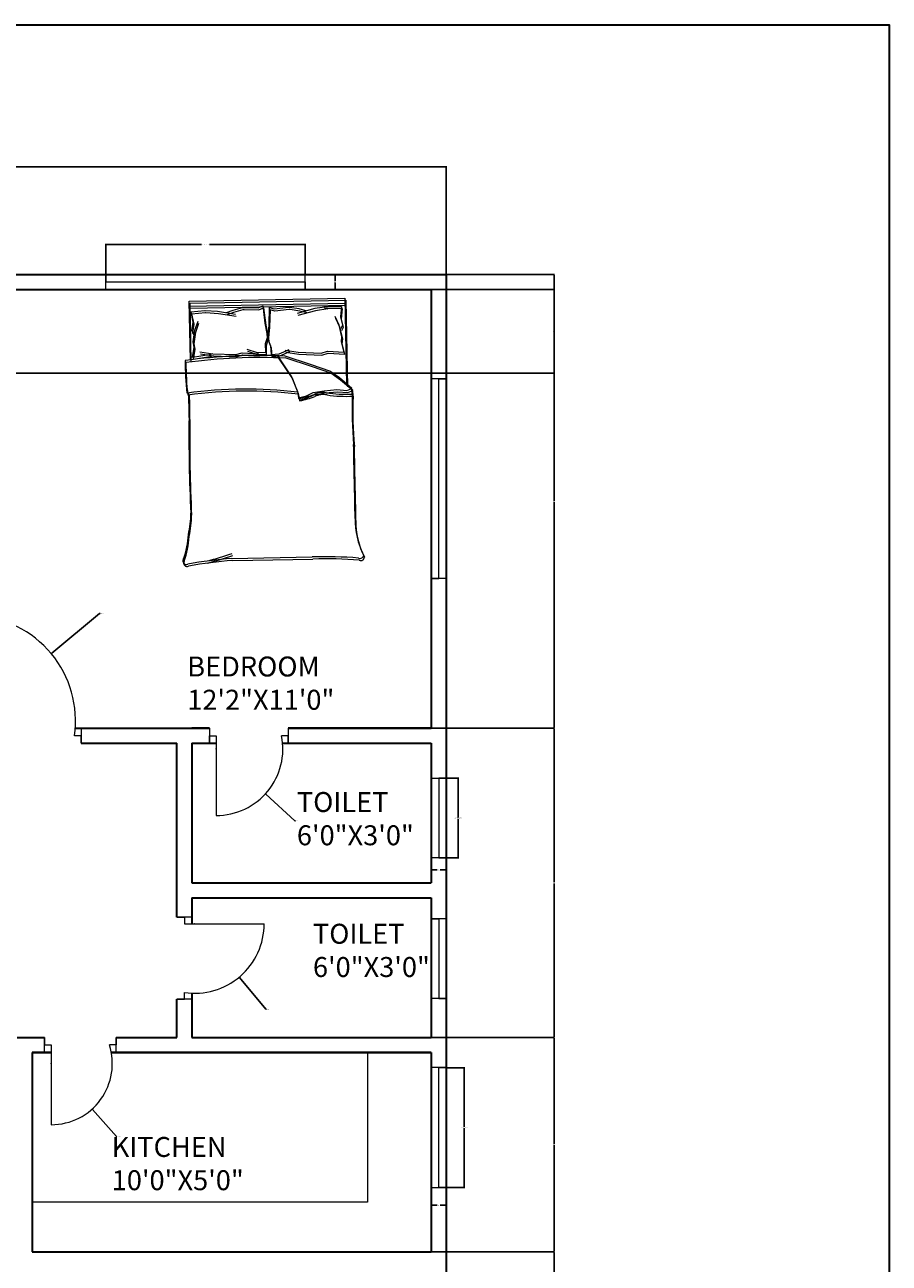
# Model space of a CAD drawing. Units: inches. Extents: x 1721 to 2510, y 1544 to 2360.
# Tile 10 of 10: x 2250 to 2510, y 1988 to 2360. Entities that reach past the tile are written whole.
import ezdxf

# ---------------------------------------------------------------- set-up
doc = ezdxf.new("R2010")
doc.units = ezdxf.units.IN
for name, color, linetype, lineweight in [('A-ANNO-DIMS', 2, 'Continuous', 18), ('A-ANNO-TTLB', 7, 'Continuous', 35), ('A-AREA-IDEN', 7, 'Continuous', 18), ('A-DOOR', 3, 'Continuous', 18), ('A-FLOR-FIXT', 9, 'Continuous', 18), ('A-FURN', 8, 'Continuous', 13), ('A-GLAZ', 4, 'Continuous', 18), ('A-WALL', 7, 'Continuous', 35)]:
    doc.layers.add(name, color=color, linetype=linetype, lineweight=lineweight)
doc.styles.get("Standard").update_dxf_attribs({"font": 'arial.ttf'})
doc.dimstyles.get("Standard").update_dxf_attribs({"dimtxt": 0.18, "dimasz": 0.18, "dimexe": 0.18, "dimexo": 0.0625, "dimgap": 0.09, "dimtad": 0, "dimtih": 1, "dimtoh": 1, "dimdec": 4, "dimzin": 0, "dimdsep": 46, "dimtxsty": 'Standard', "dimcen": 0.09, "dimadec": 0, "dimazin": 0, "dimtfac": 1, "dimtdec": 4, "dimtofl": 0, "dimtmove": 0, "dimatfit": 3, "dimfxl": 1, "dimtolj": 1, "dimtzin": 0, "dimarcsym": 0})

# ---------------------------------------------------------------- blocks, each defined once
blk = doc.blocks.new('BED-DOUBLE')
for p, q in [((39.64, 78.43), (15.52, 78.72)), ((39.64, 78.43), (15.52, 78.72)), ((39.86, 77.8), (15.74, 78.09)), ((39.86, 77.8), (15.74, 78.09)), ((1.93, 30.11), (1.99, 28.4, 3.79)), ((1.93, 30.11), (1.99, 28.4, 3.79)), ((15.66, 30.21), (13.68, 29.32)), ((15.66, 30.21), (13.68, 29.32)), ((18.1, 30.79), (15.66, 30.21)), ((18.1, 30.79), (15.66, 30.21)), ((18.31, 30.16), (15.88, 29.58)), ((18.31, 30.16), (15.88, 29.58)), ((18.38, 28.81), (18.1, 30.79)), ((18.38, 28.81), (18.1, 30.79)), ((18.59, 28.18), (18.31, 30.16)), ((18.59, 28.18), (18.31, 30.16)), ((3.5, 28.99), (1.99, 28.4)), ((3.5, 28.99), (1.99, 28.4)), ((1.99, 28.4), (5.58, 25.17)), ((1.99, 28.4), (5.58, 25.17)), ((2.15, 29.48), (2.21, 27.77, 3.79)), ((2.15, 29.48), (2.21, 27.77, 3.79)), ((3.72, 28.36), (2.21, 27.77)), ((3.72, 28.36), (2.21, 27.77)), ((2.21, 27.77), (5.8, 24.54)), ((2.21, 27.77), (5.8, 24.54)), ((3.23, 1.19), (3.55, 27.27)), ((3.23, 1.19), (3.55, 27.27)), ((3.45, 0.56), (3.76, 26.64)), ((3.45, 0.56), (3.76, 26.64)), ((6.54, 28.65), (3.5, 28.99)), ((6.54, 28.65), (3.5, 28.99)), ((6.75, 28.02), (3.72, 28.36)), ((6.75, 28.02), (3.72, 28.36)), ((10.33, 28.91), (6.54, 28.65)), ((10.33, 28.91), (6.54, 28.65)), ((10.55, 28.28), (6.75, 28.02)), ((10.55, 28.28), (6.75, 28.02)), ((13.68, 29.32), (10.33, 28.91)), ((13.68, 29.32), (10.33, 28.91)), ((13.89, 28.69), (10.55, 28.28)), ((13.89, 28.69), (10.55, 28.28)), ((15.88, 29.58), (13.89, 28.69)), ((15.88, 29.58), (13.89, 28.69)), ((20, 24.39), (18.38, 28.81)), ((20, 24.39), (18.38, 28.81)), ((20.21, 23.76), (18.59, 28.18)), ((20.21, 23.76), (18.59, 28.18)), ((5.58, 25.17), (8.44, 23.01)), ((5.58, 25.17), (8.44, 23.01)), ((5.8, 24.54), (8.66, 22.38)), ((5.8, 24.54), (8.66, 22.38)), ((8.44, 23.01), (13.88, 20.98)), ((8.44, 23.01), (13.88, 20.98)), ((8.66, 22.38), (14.1, 20.35)), ((8.66, 22.38), (14.1, 20.35)), ((24.03, 17.98), (20, 24.39)), ((24.03, 17.98), (20, 24.39)), ((24.24, 17.35), (20.21, 23.76)), ((24.24, 17.35), (20.21, 23.76)), ((13.88, 20.98), (22.02, 18)), ((13.88, 20.98), (22.02, 18)), ((14.1, 20.35), (22.24, 17.37)), ((14.1, 20.35), (22.24, 17.37)), ((9.01, 16.97), (3.98, 17.42)), ((3.98, 17.42), (4.71, 14.34)), ((9.01, 16.97), (3.98, 17.42)), ((3.98, 17.42), (4.71, 14.34)), ((9.23, 16.34), (4.2, 16.8)), ((4.2, 16.8), (4.92, 13.71)), ((9.23, 16.34), (4.2, 16.8)), ((4.2, 16.8), (4.92, 13.71)), ((10.94, 17.49), (9.01, 16.97)), ((10.94, 17.49), (9.01, 16.97)), ((11.15, 16.86), (9.23, 16.34)), ((11.15, 16.86), (9.23, 16.34)), ((17.8, 16.99), (10.94, 17.49)), ((17.8, 16.99), (10.94, 17.49)), ((18.02, 16.36), (11.15, 16.86)), ((18.02, 16.36), (11.15, 16.86)), ((21.75, 16.29), (17.8, 16.99)), ((21.75, 16.29), (17.8, 16.99)), ((21.96, 15.66), (18.02, 16.36)), ((21.96, 15.66), (18.02, 16.36)), ((23.54, 17.35), (20.51, 16.13)), ((23.54, 17.35), (20.51, 16.13)), ((23.75, 16.73), (20.73, 15.5)), ((23.75, 16.73), (20.73, 15.5)), ((25.94, 17.48), (23.54, 17.35)), ((25.94, 17.48), (23.54, 17.35)), ((26.16, 16.85), (23.75, 16.73)), ((26.16, 16.85), (23.75, 16.73)), ((26.07, 14.85), (25.94, 17.48)), ((26.07, 14.85), (25.94, 17.48)), ((26.29, 14.22), (26.16, 16.85)), ((26.29, 14.22), (26.16, 16.85)), ((27.61, 14.21), (27.64, 16.84)), ((27.61, 14.21), (27.64, 16.84)), ((27.64, 16.84), (30.05, 16.81)), ((27.64, 16.84), (30.05, 16.81)), ((27.82, 13.58), (27.85, 16.21)), ((27.82, 13.58), (27.85, 16.21)), ((27.85, 16.21), (30.26, 16.18)), ((27.85, 16.21), (30.26, 16.18)), ((34.67, 16.66), (29.65, 17.12)), ((34.67, 16.66), (29.65, 17.12)), ((34.89, 16.03), (29.86, 16.49)), ((34.89, 16.03), (29.86, 16.49)), ((30.05, 16.81), (33.11, 15.7)), ((30.05, 16.81), (33.11, 15.7)), ((30.26, 16.18), (33.33, 15.07)), ((30.26, 16.18), (33.33, 15.07)), ((36.6, 17.19), (34.67, 16.66)), ((36.6, 17.19), (34.67, 16.66)), ((36.81, 16.56), (34.89, 16.03)), ((36.81, 16.56), (34.89, 16.03)), ((43.46, 16.68), (36.6, 17.19)), ((43.46, 16.68), (36.6, 17.19)), ((43.68, 16.05), (36.81, 16.56)), ((43.68, 16.05), (36.81, 16.56)), ((43.46, 16.68), (44.58, 16.98)), ((43.46, 16.68), (44.58, 16.98)), ((47.41, 15.98), (43.46, 16.68)), ((47.41, 15.98), (43.46, 16.68)), ((43.68, 16.05), (44.79, 16.35)), ((43.68, 16.05), (44.79, 16.35)), ((47.62, 15.35), (43.68, 16.05)), ((47.62, 15.35), (43.68, 16.05)), ((44.58, 16.98), (49.58, 17.63)), ((44.58, 16.98), (49.58, 17.63)), ((44.79, 16.35), (49.8, 17)), ((44.79, 16.35), (49.8, 17)), ((49.58, 17.63), (48.98, 14.52)), ((49.58, 17.63), (48.98, 14.52)), ((49.8, 17), (49.19, 13.89)), ((49.8, 17), (49.19, 13.89)), ((50.28, 18.38), (50.07, 0.63)), ((50.28, 18.38), (50.07, 0.63)), ((50.5, 17.75), (50.29, 0)), ((50.5, 17.75), (50.29, 0)), ((4.71, 14.34), (4.5, 12.77)), ((4.71, 14.34), (4.5, 12.77)), ((4.5, 12.77), (5.25, 9.26)), ((4.5, 12.77), (5.25, 9.26)), ((4.92, 13.71), (4.72, 12.14)), ((4.92, 13.71), (4.72, 12.14)), ((4.72, 12.14), (5.46, 8.63)), ((4.72, 12.14), (5.46, 8.63)), ((26.73, 13.04), (26.07, 14.85)), ((26.73, 13.04), (26.07, 14.85)), ((26.95, 12.41), (26.29, 14.22)), ((26.95, 12.41), (26.29, 14.22)), ((26.39, 8.62), (26.8, 11.77)), ((26.39, 8.62), (26.8, 11.77)), ((26.8, 11.77), (26.73, 13.04)), ((26.8, 11.77), (26.73, 13.04)), ((27.01, 11.14), (26.95, 12.41)), ((27.01, 11.14), (26.95, 12.41)), ((27, 11.1), (27.02, 12.38)), ((27, 11.1), (27.02, 12.38)), ((27.02, 12.38), (27.61, 14.21)), ((27.02, 12.38), (27.61, 14.21)), ((27.22, 10.47), (27.23, 11.75)), ((27.22, 10.47), (27.23, 11.75)), ((27.23, 11.75), (27.82, 13.58)), ((27.23, 11.75), (27.82, 13.58)), ((49.24, 12.96), (48.63, 9.42)), ((49.24, 12.96), (48.63, 9.42)), ((49.46, 12.33), (48.85, 8.79)), ((49.46, 12.33), (48.85, 8.79)), ((48.98, 14.52), (49.24, 12.96)), ((48.98, 14.52), (49.24, 12.96)), ((49.19, 13.89), (49.46, 12.33)), ((49.19, 13.89), (49.46, 12.33)), ((4.25, 9.35), (4.77, 10.37)), ((4.25, 9.35), (4.77, 10.37)), ((4.8, 6.82), (4.25, 9.35)), ((4.8, 6.82), (4.25, 9.35)), ((4.47, 8.72), (4.98, 9.74)), ((4.47, 8.72), (4.98, 9.74)), ((5.02, 6.19), (4.47, 8.72)), ((5.02, 6.19), (4.47, 8.72)), ((5.25, 9.26), (6.37, 6.62)), ((5.25, 9.26), (6.37, 6.62)), ((5.46, 8.63), (6.59, 5.99)), ((5.46, 8.63), (6.59, 5.99)), ((26.09, 3.36), (26.39, 8.62)), ((26.09, 3.36), (26.39, 8.62)), ((26.3, 2.73), (26.61, 7.99)), ((26.3, 2.73), (26.61, 7.99)), ((26.61, 7.99), (27.01, 11.14)), ((26.61, 7.99), (27.01, 11.14)), ((27.53, 7.98), (27, 11.1)), ((27.53, 7.98), (27, 11.1)), ((27.75, 7.35), (27.22, 10.47)), ((27.75, 7.35), (27.22, 10.47)), ((28.04, 2.73), (27.53, 7.98)), ((28.04, 2.73), (27.53, 7.98)), ((48.63, 9.42), (47.61, 6.74)), ((48.63, 9.42), (47.61, 6.74)), ((48.85, 8.79), (47.82, 6.11)), ((48.85, 8.79), (47.82, 6.11)), ((49.63, 9.55), (49.07, 10.55)), ((49.63, 9.55), (49.07, 10.55)), ((49.17, 7.01), (49.63, 9.55)), ((49.17, 7.01), (49.63, 9.55)), ((49.84, 8.92), (49.29, 9.92)), ((49.84, 8.92), (49.29, 9.92)), ((49.39, 6.38), (49.84, 8.92)), ((49.39, 6.38), (49.84, 8.92)), ((4.39, 3.68), (4.8, 6.82)), ((4.39, 3.68), (4.8, 6.82)), ((4.61, 3.05), (5.02, 6.19)), ((4.61, 3.05), (5.02, 6.19)), ((8.71, 3.62), (12.44, 4.09)), ((8.71, 3.62), (12.44, 4.09)), ((12.44, 4.09), (17.76, 5.35)), ((12.44, 4.09), (17.76, 5.35)), ((12.65, 3.46), (17.98, 4.72)), ((12.65, 3.46), (17.98, 4.72)), ((15.1, 4.65), (17.12, 4.04)), ((15.1, 4.65), (17.12, 4.04)), ((15.32, 4.02), (17.34, 3.41)), ((15.32, 4.02), (17.34, 3.41)), ((17.12, 4.04), (19.98, 3.48)), ((17.12, 4.04), (19.98, 3.48)), ((20.3, 3.49), (24.64, 3.85)), ((20.3, 3.49), (24.64, 3.85)), ((24.64, 3.85), (26.09, 3.36)), ((24.64, 3.85), (26.09, 3.36)), ((28.25, 2.1), (27.75, 7.35)), ((28.25, 2.1), (27.75, 7.35)), ((36.97, 3.75), (34.13, 3.08)), ((36.97, 3.75), (34.13, 3.08)), ((41.65, 3.98), (36.28, 5.04)), ((41.65, 3.98), (36.28, 5.04)), ((41.87, 3.35), (36.49, 4.41)), ((41.87, 3.35), (36.49, 4.41)), ((38.96, 4.44), (36.97, 3.75)), ((38.96, 4.44), (36.97, 3.75)), ((39.18, 3.81), (37.19, 3.12)), ((39.18, 3.81), (37.19, 3.12)), ((45.39, 3.65), (41.65, 3.98)), ((45.39, 3.65), (41.65, 3.98)), ((49.7, 3.91), (45.5, 3.63)), ((49.7, 3.91), (45.5, 3.63)), ((49.7, 3.88), (49.17, 7.01)), ((49.7, 3.88), (49.17, 7.01)), ((49.92, 3.25), (49.39, 6.38)), ((49.92, 3.25), (49.39, 6.38)), ((50.07, 0.63), (3.23, 1.19)), ((50.07, 0.63), (3.23, 1.19)), ((50.09, 2.13), (3.25, 2.69)), ((50.09, 2.13), (3.25, 2.69)), ((50.29, 0), (3.45, 0.56)), ((50.29, 0), (3.45, 0.56)), ((50.31, 1.5), (3.47, 2.06)), ((50.31, 1.5), (3.47, 2.06)), ((4.39, 3.68), (9.69, 3.52)), ((4.39, 3.68), (9.69, 3.52)), ((4.61, 3.05), (9.9, 2.89)), ((4.61, 3.05), (9.9, 2.89)), ((9.69, 3.52), (8.71, 3.62)), ((9.69, 3.52), (8.71, 3.62)), ((8.92, 2.99), (12.65, 3.46)), ((8.92, 2.99), (12.65, 3.46)), ((9.9, 2.89), (8.92, 2.99)), ((9.9, 2.89), (8.92, 2.99)), ((17.34, 3.41), (20.2, 2.85)), ((17.34, 3.41), (20.2, 2.85)), ((19.98, 3.48), (20.3, 3.49)), ((19.98, 3.48), (20.3, 3.49)), ((20.2, 2.85), (20.52, 2.86)), ((20.2, 2.85), (20.52, 2.86)), ((20.52, 2.86), (24.86, 3.22)), ((20.52, 2.86), (24.86, 3.22)), ((24.86, 3.22), (26.3, 2.73)), ((24.86, 3.22), (26.3, 2.73)), ((29.46, 3.28), (28.04, 2.73)), ((29.46, 3.28), (28.04, 2.73)), ((29.68, 2.65), (28.25, 2.1)), ((29.68, 2.65), (28.25, 2.1)), ((33.81, 3.08), (29.46, 3.28)), ((33.81, 3.08), (29.46, 3.28)), ((34.03, 2.45), (29.68, 2.65)), ((34.03, 2.45), (29.68, 2.65)), ((34.13, 3.08), (33.81, 3.08)), ((34.13, 3.08), (33.81, 3.08)), ((34.35, 2.45), (34.03, 2.45)), ((34.35, 2.45), (34.03, 2.45)), ((37.19, 3.12), (34.35, 2.45)), ((37.19, 3.12), (34.35, 2.45)), ((45.61, 3.02), (41.87, 3.35)), ((45.61, 3.02), (41.87, 3.35)), ((45.5, 3.63), (45.39, 3.65)), ((45.5, 3.63), (45.39, 3.65)), ((45.71, 3), (45.61, 3.02)), ((45.71, 3), (45.61, 3.02)), ((49.91, 3.28), (45.71, 3)), ((49.91, 3.28), (45.71, 3))]:
    blk.add_line(p, q)
for centre, radius, start, end in [((1.08, 78.52), 1.08, 61.9736, 175.3348), ((1.08, 78.52), 1.08, 61.9736, 175.3348), ((-20.36, 68.78), 22.61, 356.7862, 25.7829), ((-20.36, 68.78), 22.61, 356.7862, 25.7829), ((1.29, 77.89), 1.08, 61.9736, 175.3348), ((1.29, 77.89), 1.08, 61.9736, 175.3348), ((15.63, 209.12), 130.4, 263.8146, 269.9499), ((15.63, 209.12), 130.4, 263.8146, 269.9499), ((15.85, 208.49), 130.4, 263.8146, 269.9499), ((15.85, 208.49), 130.4, 263.8146, 269.9499), ((70.08, -22.85), 104.34, 102.698, 107.0202), ((70.08, -22.85), 104.34, 102.698, 107.0202), ((34.83, 197.67), 119.34, 272.3106, 278.7239), ((34.83, 197.67), 119.34, 272.3106, 278.7239), ((70.29, -23.48), 104.34, 102.698, 107.0202), ((70.29, -23.48), 104.34, 102.698, 107.0202), ((35.05, 197.04), 119.34, 272.3106, 278.7239), ((35.05, 197.04), 119.34, 272.3106, 278.7239), ((53.35, 78.73), 1.07, 325.4884, 112.793), ((53.35, 78.73), 1.07, 325.4884, 112.793), ((53.56, 78.1), 1.07, 325.4884, 112.793), ((53.56, 78.1), 1.07, 325.4884, 112.793), ((-20.14, 68.15), 22.61, 356.7862, 25.7829), ((-20.14, 68.15), 22.61, 356.7862, 25.7829), ((75.53, 69.21), 23.09, 157.2899, 175.9668), ((75.53, 69.21), 23.09, 157.2899, 175.9668), ((75.75, 68.58), 23.09, 157.2899, 175.9668), ((75.75, 68.58), 23.09, 157.2899, 175.9668), ((80.6, 63.5), 29.05, 165.3797, 178.2261), ((80.6, 63.5), 29.05, 165.3797, 178.2261), ((4473.12, 14.21), 4471.22, 179.317, 179.60172), ((4473.12, 14.21), 4471.22, 179.317, 179.60172), ((80.81, 62.87), 29.05, 165.3797, 178.2261), ((80.81, 62.87), 29.05, 165.3797, 178.2261), ((4473.34, 13.58), 4471.22, 179.317, 179.60172), ((4473.34, 13.58), 4471.22, 179.317, 179.60172), ((-421.08, 55.88), 472.73, 357.5425, 1.0334), ((-421.08, 55.88), 472.73, 357.5425, 1.0334), ((-420.87, 55.25), 472.73, 357.5425, 1.0334), ((-420.87, 55.25), 472.73, 357.5425, 1.0334), ((-124.73, 38.32), 126.93, 356.294, 3.1513), ((-124.73, 38.32), 126.93, 356.294, 3.1513), ((-124.51, 37.69), 126.93, 356.294, 3.1513), ((-124.51, 37.69), 126.93, 356.294, 3.1513), ((217.81, 29.18), 166.73, 177.791, 180.323), ((217.81, 29.18), 166.73, 177.791, 180.323), ((218.03, 28.55), 166.73, 177.791, 180.323), ((218.03, 28.55), 166.73, 177.791, 180.323), ((3.1, -5.33), 35.46, 79.1911, 91.8805), ((3.1, -5.33), 35.46, 79.1911, 91.8805), ((11.02, 35.47), 6.1, 257.9756, 293.0532), ((11.02, 35.47), 6.1, 257.9756, 293.0532), ((22.96, 2.41), 29.06, 99.9765, 109.1954), ((22.96, 2.41), 29.06, 99.9765, 109.1954), ((23.18, 1.78), 29.06, 99.9765, 109.1954), ((23.18, 1.78), 29.06, 99.9765, 109.1954), ((17.93, 30.85), 0.181, 339.5612, 90.4525), ((17.93, 30.85), 0.181, 339.5612, 90.4525), ((18.15, 30.22), 0.181, 339.5612, 90.4525), ((18.15, 30.22), 0.181, 339.5612, 90.4525), ((3.31, -5.96), 35.46, 79.1911, 91.8805), ((3.31, -5.96), 35.46, 79.1911, 91.8805), ((11.23, 34.84), 6.1, 257.9756, 293.0532), ((11.23, 34.84), 6.1, 257.9756, 293.0532), ((37.91, 154), 126.46, 261.0993, 276.2154), ((37.91, 154), 126.46, 261.0993, 276.2154), ((38.12, 153.37), 126.46, 261.0993, 276.2154), ((38.12, 153.37), 126.46, 261.0993, 276.2154), ((-29.75, 21.28), 81.65, 358.0366, 4.9188), ((-29.75, 21.28), 81.65, 358.0366, 4.9188), ((-29.53, 20.65), 81.65, 358.0366, 4.9188), ((-29.53, 20.65), 81.65, 358.0366, 4.9188), ((34.68, 179.26), 161.69, 265.4014, 276.097), ((34.68, 179.26), 161.69, 265.4014, 276.097), ((34.89, 178.63), 161.69, 265.4014, 276.097), ((34.89, 178.63), 161.69, 265.4014, 276.097)]:
    blk.add_arc(centre, radius, start, end)
blk = doc.blocks.new('WIN-60IN-A')
for p, q in [((4.5, 60), (0, 60)), ((2.25, 0), (2.25, 60)), ((2.25, 60), (4.5, 60)), ((4.5, 0), (0, 0)), ((0, 0), (2.25, 0))]:
    blk.add_line(p, q)
blk = doc.blocks.new('WIN-24IN-A')
for p, q in [((4.5, 24), (0, 24)), ((0, 24), (2.25, 24)), ((2.25, 24), (2.25, 0)), ((4.5, 0), (0, 0)), ((2.25, 0), (4.5, 0))]:
    blk.add_line(p, q)
blk = doc.blocks.new('WIN-24IN-B')
for p, q in [((0, 24), (4.5, 24)), ((4.5, 24), (2.25, 24)), ((2.25, 24), (2.25, 0)), ((4.5, 0), (0, 0)), ((2.25, 0), (4.5, 0))]:
    blk.add_line(p, q)
blk = doc.blocks.new('WIN-36IN-B')
for p, q in [((4.5, 36), (0, 36)), ((2.25, 0), (2.25, 36)), ((2.25, 36), (4.5, 36)), ((0, 0), (4.5, 0)), ((4.5, 0), (2.25, 0))]:
    blk.add_line(p, q)
blk = doc.blocks.new('*D18')
at = {"layer": 'A-ANNO-DIMS', "color": 0, "lineweight": -2, "transparency": 16777216}
for p, q in [((2274.1, 2285.19), (2274.1, 2294.31)), ((2274.28, 2294.13), (2302.86, 2294.13)), ((2333.92, 2294.13), (2305.33, 2294.13)), ((2334.1, 2285.19), (2334.1, 2294.31))]:
    blk.add_line(p, q, dxfattribs=at)
at = {"layer": 'A-ANNO-DIMS', "color": 0, "transparency": 16777216}
for points in [[(2274.28, 2294.16), (2274.28, 2294.1), (2274.1, 2294.13)], [(2333.92, 2294.16), (2333.92, 2294.1), (2334.1, 2294.13)]]:
    blk.add_solid(points, dxfattribs=at)
at = {"layer": 'Defpoints', "color": 0, "transparency": 16777216}
for p in [(2334.1, 2294.13), (2274.1, 2285.13), (2334.1, 2285.13)]:
    blk.add_point(p, dxfattribs=at)
at = {"layer": 'A-ANNO-DIMS', "color": 0, "transparency": 16777216, "insert": (2304.1, 2294.13), "char_height": 0.18, "attachment_point": 5}
blk.add_mtext('\\A1;WINDOW A 60 TYP.', dxfattribs=at)
blk = doc.blocks.new('*D19')
at = {"layer": 'A-ANNO-DIMS', "color": 0, "lineweight": -2, "transparency": 16777216}
for p, q in [((2334.16, 2285.13), (2343.28, 2285.13)), ((2343.1, 2284.95), (2343.1, 2283.06)), ((2334.16, 2280.63), (2343.28, 2280.63)), ((2343.1, 2280.81), (2343.1, 2282.7))]:
    blk.add_line(p, q, dxfattribs=at)
at = {"layer": 'A-ANNO-DIMS', "color": 0, "transparency": 16777216}
for points in [[(2343.07, 2284.95), (2343.13, 2284.95), (2343.1, 2285.13)], [(2343.07, 2280.81), (2343.13, 2280.81), (2343.1, 2280.63)]]:
    blk.add_solid(points, dxfattribs=at)
at = {"layer": 'Defpoints', "color": 0, "transparency": 16777216}
for p in [(2334.1, 2285.13), (2334.1, 2280.63), (2343.1, 2280.63)]:
    blk.add_point(p, dxfattribs=at)
at = {"layer": 'A-ANNO-DIMS', "color": 0, "transparency": 16777216, "insert": (2343.1, 2282.88), "char_height": 0.18, "attachment_point": 5}
blk.add_mtext('\\A1;5 TYP.', dxfattribs=at)
blk = doc.blocks.new('*D24')
at = {"layer": 'A-ANNO-DIMS', "color": 0, "lineweight": -2, "transparency": 16777216}
for p, q in [((2376.56, 2046.53), (2382.08, 2046.53)), ((2381.9, 2046.35), (2381.9, 2028.72)), ((2381.9, 2010.71), (2381.9, 2028.35)), ((2376.56, 2010.53), (2382.08, 2010.53))]:
    blk.add_line(p, q, dxfattribs=at)
at = {"layer": 'A-ANNO-DIMS', "color": 0, "transparency": 16777216}
for points in [[(2381.87, 2046.35), (2381.93, 2046.35), (2381.9, 2046.53)], [(2381.87, 2010.71), (2381.93, 2010.71), (2381.9, 2010.53)]]:
    blk.add_solid(points, dxfattribs=at)
at = {"layer": 'Defpoints', "color": 0, "transparency": 16777216}
for p in [(2376.5, 2046.53), (2381.9, 2046.53), (2376.5, 2010.53)]:
    blk.add_point(p, dxfattribs=at)
at = {"layer": 'A-ANNO-DIMS', "color": 0, "transparency": 16777216, "insert": (2381.9, 2028.53), "char_height": 0.18, "attachment_point": 5}
blk.add_mtext('\\A1;WINDOW B 36 TYP.', dxfattribs=at)
blk = doc.blocks.new('*D25')
at = {"layer": 'A-ANNO-DIMS', "color": 0, "lineweight": -2, "transparency": 16777216}
for p, q in [((2372, 2010.47), (2372, 2004.95)), ((2376.5, 2010.47), (2376.5, 2004.95)), ((2372.18, 2005.13), (2373.79, 2005.13)), ((2376.32, 2005.13), (2374.71, 2005.13))]:
    blk.add_line(p, q, dxfattribs=at)
at = {"layer": 'A-ANNO-DIMS', "color": 0, "transparency": 16777216}
for points in [[(2372.18, 2005.16), (2372.18, 2005.1), (2372, 2005.13)], [(2376.32, 2005.16), (2376.32, 2005.1), (2376.5, 2005.13)]]:
    blk.add_solid(points, dxfattribs=at)
at = {"layer": 'Defpoints', "color": 0, "transparency": 16777216}
for p in [(2372, 2010.53), (2376.5, 2010.53), (2376.5, 2005.13)]:
    blk.add_point(p, dxfattribs=at)
at = {"layer": 'A-ANNO-DIMS', "color": 0, "transparency": 16777216, "insert": (2374.25, 2005.13), "char_height": 0.18, "attachment_point": 5}
blk.add_mtext('\\A1;5 TYP.', dxfattribs=at)
blk = doc.blocks.new('*D28')
at = {"layer": 'A-ANNO-DIMS', "color": 0, "lineweight": -2, "transparency": 16777216}
for p, q in [((2376.56, 2133.6), (2380.28, 2133.6)), ((2380.1, 2133.42), (2380.1, 2121.78)), ((2380.1, 2109.78), (2380.1, 2121.42)), ((2376.56, 2109.6), (2380.28, 2109.6))]:
    blk.add_line(p, q, dxfattribs=at)
at = {"layer": 'A-ANNO-DIMS', "color": 0, "transparency": 16777216}
for points in [[(2380.07, 2133.42), (2380.13, 2133.42), (2380.1, 2133.6)], [(2380.07, 2109.78), (2380.13, 2109.78), (2380.1, 2109.6)]]:
    blk.add_solid(points, dxfattribs=at)
at = {"layer": 'Defpoints', "color": 0, "transparency": 16777216}
for p in [(2376.5, 2133.6), (2380.1, 2133.6), (2376.5, 2109.6)]:
    blk.add_point(p, dxfattribs=at)
at = {"layer": 'A-ANNO-DIMS', "color": 0, "transparency": 16777216, "insert": (2380.1, 2121.6), "char_height": 0.18, "attachment_point": 5}
blk.add_mtext('\\A1;WINDOW B 24 TYP.', dxfattribs=at)
blk = doc.blocks.new('*D29')
at = {"layer": 'A-ANNO-DIMS', "color": 0, "lineweight": -2, "transparency": 16777216}
for p, q in [((2372, 2109.54), (2372, 2105.82)), ((2376.5, 2109.54), (2376.5, 2105.82)), ((2372.18, 2106), (2373.79, 2106)), ((2376.32, 2106), (2374.71, 2106))]:
    blk.add_line(p, q, dxfattribs=at)
at = {"layer": 'A-ANNO-DIMS', "color": 0, "transparency": 16777216}
for points in [[(2372.18, 2106.03), (2372.18, 2105.97), (2372, 2106)], [(2376.32, 2106.03), (2376.32, 2105.97), (2376.5, 2106)]]:
    blk.add_solid(points, dxfattribs=at)
at = {"layer": 'Defpoints', "color": 0, "transparency": 16777216}
for p in [(2372, 2109.6), (2376.5, 2109.6), (2376.5, 2106)]:
    blk.add_point(p, dxfattribs=at)
at = {"layer": 'A-ANNO-DIMS', "color": 0, "transparency": 16777216, "insert": (2374.25, 2106), "char_height": 0.18, "attachment_point": 5}
blk.add_mtext('\\A1;5 TYP.', dxfattribs=at)
blk = doc.blocks.new('*D40')
at = {"layer": 'A-ANNO-DIMS', "color": 0, "lineweight": -2, "transparency": 16777216}
for p, q in [((1798, 2285.19), (1798, 2317.71)), ((1798.18, 2317.53), (2086.86, 2317.53)), ((2376.32, 2317.53), (2087.65, 2317.53)), ((2376.5, 2285.19), (2376.5, 2317.71))]:
    blk.add_line(p, q, dxfattribs=at)
at = {"layer": 'A-ANNO-DIMS', "color": 0, "transparency": 16777216}
for points in [[(1798.18, 2317.56), (1798.18, 2317.5), (1798, 2317.53)], [(2376.32, 2317.56), (2376.32, 2317.5), (2376.5, 2317.53)]]:
    blk.add_solid(points, dxfattribs=at)
at = {"layer": 'Defpoints', "color": 0, "transparency": 16777216}
for p in [(2376.5, 2317.53), (1798, 2285.13), (2376.5, 2285.13)]:
    blk.add_point(p, dxfattribs=at)
at = {"layer": 'A-ANNO-DIMS', "color": 0, "transparency": 16777216, "insert": (2087.25, 2317.53), "char_height": 0.18, "attachment_point": 5}
blk.add_mtext('\\A1;578.5', dxfattribs=at)
blk = doc.blocks.new('*D47')
at = {"layer": 'A-ANNO-DIMS', "color": 0, "lineweight": -2, "transparency": 16777216}
for p, q in [((2376.56, 2285.13), (2409.08, 2285.13)), ((2408.9, 2284.95), (2408.9, 2217.06)), ((2408.9, 2148.81), (2408.9, 2216.7)), ((2372.06, 2148.63), (2409.08, 2148.63))]:
    blk.add_line(p, q, dxfattribs=at)
at = {"layer": 'A-ANNO-DIMS', "color": 0, "transparency": 16777216}
for points in [[(2408.87, 2284.95), (2408.93, 2284.95), (2408.9, 2285.13)], [(2408.87, 2148.81), (2408.93, 2148.81), (2408.9, 2148.63)]]:
    blk.add_solid(points, dxfattribs=at)
at = {"layer": 'Defpoints', "color": 0, "transparency": 16777216}
for p in [(2376.5, 2285.13), (2408.9, 2285.13), (2372, 2148.63)]:
    blk.add_point(p, dxfattribs=at)
at = {"layer": 'A-ANNO-DIMS', "color": 0, "transparency": 16777216, "insert": (2408.9, 2216.88), "char_height": 0.18, "attachment_point": 5}
blk.add_mtext('\\A1;136.5', dxfattribs=at)
blk = doc.blocks.new('*D48')
at = {"layer": 'A-ANNO-DIMS', "color": 0, "lineweight": -2, "transparency": 16777216}
for p, q in [((2372.06, 2148.63), (2409.08, 2148.63)), ((2408.9, 2148.45), (2408.9, 2102.31)), ((2408.9, 2055.81), (2408.9, 2101.95)), ((2372.06, 2055.63), (2409.08, 2055.63))]:
    blk.add_line(p, q, dxfattribs=at)
at = {"layer": 'A-ANNO-DIMS', "color": 0, "transparency": 16777216}
for points in [[(2408.87, 2148.45), (2408.93, 2148.45), (2408.9, 2148.63)], [(2408.87, 2055.81), (2408.93, 2055.81), (2408.9, 2055.63)]]:
    blk.add_solid(points, dxfattribs=at)
at = {"layer": 'Defpoints', "color": 0, "transparency": 16777216}
for p in [(2372, 2148.63), (2408.9, 2148.63), (2372, 2055.63)]:
    blk.add_point(p, dxfattribs=at)
at = {"layer": 'A-ANNO-DIMS', "color": 0, "transparency": 16777216, "insert": (2408.9, 2102.13), "char_height": 0.18, "attachment_point": 5}
blk.add_mtext('\\A1;93', dxfattribs=at)
blk = doc.blocks.new('*D49')
at = {"layer": 'A-ANNO-DIMS', "color": 0, "lineweight": -2, "transparency": 16777216}
for p, q in [((2372.06, 2055.63), (2409.08, 2055.63)), ((2408.9, 2055.45), (2408.9, 2023.56)), ((2408.9, 1991.31), (2408.9, 2023.2)), ((2372.06, 1991.13), (2409.08, 1991.13))]:
    blk.add_line(p, q, dxfattribs=at)
at = {"layer": 'A-ANNO-DIMS', "color": 0, "transparency": 16777216}
for points in [[(2408.87, 2055.45), (2408.93, 2055.45), (2408.9, 2055.63)], [(2408.87, 1991.31), (2408.93, 1991.31), (2408.9, 1991.13)]]:
    blk.add_solid(points, dxfattribs=at)
at = {"layer": 'Defpoints', "color": 0, "transparency": 16777216}
for p in [(2372, 2055.63), (2408.9, 2055.63), (2372, 1991.13)]:
    blk.add_point(p, dxfattribs=at)
at = {"layer": 'A-ANNO-DIMS', "color": 0, "transparency": 16777216, "insert": (2408.9, 2023.38), "char_height": 0.18, "attachment_point": 5}
blk.add_mtext('\\A1;64.5', dxfattribs=at)
blk = doc.blocks.new('*D50')
at = {"layer": 'A-ANNO-DIMS', "color": 0, "lineweight": -2, "transparency": 16777216}
for p, q in [((2372.06, 1991.13), (2409.08, 1991.13)), ((2408.9, 1990.95), (2408.9, 1959.06)), ((2408.9, 1926.81), (2408.9, 1958.7)), ((2372.06, 1926.63), (2409.08, 1926.63))]:
    blk.add_line(p, q, dxfattribs=at)
at = {"layer": 'A-ANNO-DIMS', "color": 0, "transparency": 16777216}
for points in [[(2408.87, 1990.95), (2408.93, 1990.95), (2408.9, 1991.13)], [(2408.87, 1926.81), (2408.93, 1926.81), (2408.9, 1926.63)]]:
    blk.add_solid(points, dxfattribs=at)
at = {"layer": 'Defpoints', "color": 0, "transparency": 16777216}
for p in [(2372, 1991.13), (2408.9, 1991.13), (2372, 1926.63)]:
    blk.add_point(p, dxfattribs=at)
at = {"layer": 'A-ANNO-DIMS', "color": 0, "transparency": 16777216, "insert": (2408.9, 1958.88), "char_height": 0.18, "attachment_point": 5}
blk.add_mtext('\\A1;64.5', dxfattribs=at)
blk = doc.blocks.new('*D57')
at = {"layer": 'A-ANNO-DIMS', "color": 0, "lineweight": -2, "transparency": 16777216}
for p, q in [((1802.56, 2280.63), (2409.08, 2280.63)), ((2408.9, 2280.45), (2408.9, 2268.22)), ((2408.9, 2255.63), (2408.9, 2267.86)), ((1802.56, 2255.45), (2409.08, 2255.45))]:
    blk.add_line(p, q, dxfattribs=at)
at = {"layer": 'A-ANNO-DIMS', "color": 0, "transparency": 16777216}
for points in [[(2408.87, 2280.45), (2408.93, 2280.45), (2408.9, 2280.63)], [(2408.87, 2255.63), (2408.93, 2255.63), (2408.9, 2255.45)]]:
    blk.add_solid(points, dxfattribs=at)
at = {"layer": 'Defpoints', "color": 0, "transparency": 16777216}
for p in [(1802.5, 2280.63), (1802.5, 2255.45), (2408.9, 2255.45)]:
    blk.add_point(p, dxfattribs=at)
at = {"layer": 'A-ANNO-DIMS', "color": 0, "transparency": 16777216, "insert": (2408.9, 2268.04), "char_height": 0.18, "attachment_point": 5}
blk.add_mtext('\\A1;25.18', dxfattribs=at)
blk = doc.blocks.new('*D76')
at = {"layer": 'A-ANNO-DIMS', "color": 0, "lineweight": -2, "transparency": 16777216}
for p, q in [((2272.21, 2183.16), (2257.85, 2171.2)), ((2272.39, 2183.16), (2272.21, 2183.16)), ((2233.46, 2150.95), (2233.64, 2150.95)), ((2233.55, 2150.86), (2233.55, 2151.04))]:
    blk.add_line(p, q, dxfattribs=at)
at = {"layer": 'A-ANNO-DIMS', "color": 0, "transparency": 16777216}
blk.add_solid([(2257.83, 2171.22), (2257.87, 2171.17), (2257.71, 2171.08)], dxfattribs=at)
at = {"layer": 'Defpoints', "color": 0, "transparency": 16777216}
for p in [(2257.71, 2171.08), (2233.55, 2150.95)]:
    blk.add_point(p, dxfattribs=at)
at = {"layer": 'A-ANNO-DIMS', "color": 0, "transparency": 16777216, "insert": (2272.93, 2183.16), "char_height": 0.18, "attachment_point": 5}
blk.add_mtext('\\A1;R31.446', dxfattribs=at)
blk = doc.blocks.new('*D88')
at = {"layer": 'A-ANNO-DIMS', "color": 0, "lineweight": -2, "transparency": 16777216}
for p, q in [((2307.23, 2142.44), (2307.41, 2142.44)), ((2307.32, 2142.35), (2307.32, 2142.53)), ((2330.99, 2120.77), (2322.25, 2128.77)), ((2331.17, 2120.77), (2330.99, 2120.77))]:
    blk.add_line(p, q, dxfattribs=at)
at = {"layer": 'A-ANNO-DIMS', "color": 0, "transparency": 16777216}
blk.add_solid([(2322.27, 2128.8), (2322.23, 2128.75), (2322.11, 2128.9)], dxfattribs=at)
at = {"layer": 'Defpoints', "color": 0, "transparency": 16777216}
for p in [(2307.32, 2142.44), (2322.11, 2128.9)]:
    blk.add_point(p, dxfattribs=at)
at = {"layer": 'A-ANNO-DIMS', "color": 0, "transparency": 16777216, "insert": (2331.72, 2120.77), "char_height": 0.18, "attachment_point": 5}
blk.add_mtext('\\A1;R20.057', dxfattribs=at)
blk = doc.blocks.new('*D89')
at = {"layer": 'A-ANNO-DIMS', "color": 0, "lineweight": -2, "transparency": 16777216}
for p, q in [((2300.75, 2089.83), (2300.93, 2089.83)), ((2300.84, 2089.74), (2300.84, 2089.92)), ((2322.23, 2064.1), (2314.32, 2073.61)), ((2322.41, 2064.1), (2322.23, 2064.1))]:
    blk.add_line(p, q, dxfattribs=at)
at = {"layer": 'A-ANNO-DIMS', "color": 0, "transparency": 16777216}
blk.add_solid([(2314.35, 2073.63), (2314.3, 2073.59), (2314.21, 2073.75)], dxfattribs=at)
at = {"layer": 'Defpoints', "color": 0, "transparency": 16777216}
for p in [(2300.84, 2089.83), (2314.21, 2073.75)]:
    blk.add_point(p, dxfattribs=at)
at = {"layer": 'A-ANNO-DIMS', "color": 0, "transparency": 16777216, "insert": (2322.87, 2064.1), "char_height": 0.18, "attachment_point": 5}
blk.add_mtext('\\A1;R20.91', dxfattribs=at)
blk = doc.blocks.new('*D90')
at = {"layer": 'A-ANNO-DIMS', "color": 0, "lineweight": -2, "transparency": 16777216}
for p, q in [((2257.63, 2047.75), (2257.81, 2047.75)), ((2257.72, 2047.66), (2257.72, 2047.84)), ((2277.3, 2025.83), (2270.07, 2033.92)), ((2277.48, 2025.83), (2277.3, 2025.83))]:
    blk.add_line(p, q, dxfattribs=at)
at = {"layer": 'A-ANNO-DIMS', "color": 0, "transparency": 16777216}
blk.add_solid([(2270.1, 2033.94), (2270.05, 2033.9), (2269.95, 2034.05)], dxfattribs=at)
at = {"layer": 'Defpoints', "color": 0, "transparency": 16777216}
for p in [(2257.72, 2047.75), (2269.95, 2034.05)]:
    blk.add_point(p, dxfattribs=at)
at = {"layer": 'A-ANNO-DIMS', "color": 0, "transparency": 16777216, "insert": (2278.03, 2025.83), "char_height": 0.18, "attachment_point": 5}
blk.add_mtext('\\A1;R18.365', dxfattribs=at)

msp = doc.modelspace()

# ---------------------------------------------------------------- linework, layer by layer
at = {"layer": 'A-ANNO-TTLB'}
msp.add_lwpolyline([(1721.1268, 2360.2177), (2509.707, 2360.2177), (2509.707, 1544.3037), (1721.1268, 1544.3037)], close=True, dxfattribs=at)
at = {"layer": 'A-DOOR'}
for p, q in [((2266.6606, 2146.3798), (2264.6606, 2146.3798)), ((2266.6606, 2148.6298), (2266.6606, 2144.1298)), ((2266.6606, 2144.1298), (2266.6606, 2146.3798)), ((2305.3168, 2148.6298), (2305.3168, 2144.1298)), ((2305.3168, 2144.1298), (2305.3168, 2146.3798)), ((2305.3168, 2146.3798), (2307.3168, 2146.3798)), ((2307.3168, 2146.3798), (2307.3168, 2122.3798)), ((2328.9823, 2146.3798), (2326.9823, 2146.3798)), ((2328.9823, 2148.6298), (2328.9823, 2144.1298)), ((2328.9823, 2144.1298), (2328.9823, 2146.3798)), ((2300.0024, 2091.8314), (2295.5024, 2091.8314)), ((2295.5024, 2091.8314), (2297.7524, 2091.8314)), ((2297.7524, 2091.8314), (2297.7524, 2089.8314)), ((2297.7524, 2089.8314), (2321.7524, 2089.8314)), ((2297.7524, 2067.1507), (2297.7524, 2069.1507)), ((2300.0024, 2067.1507), (2295.5024, 2067.1507)), ((2295.5024, 2067.1507), (2297.7524, 2067.1507)), ((2255.717, 2051.1298), (2255.717, 2055.6298)), ((2255.717, 2055.6298), (2255.717, 2053.3798)), ((2255.717, 2053.3798), (2257.717, 2053.3798)), ((2257.717, 2053.3798), (2257.717, 2029.3798)), ((2277.1967, 2053.3798), (2275.1967, 2053.3798)), ((2277.1967, 2051.1298), (2277.1967, 2055.6298)), ((2277.1967, 2055.6298), (2277.1967, 2053.3798))]:
    msp.add_line(p, q, dxfattribs=at)
for centre, radius, start, end in [((2233.549, 2150.9538), 31.446, 351.636388, 87.958091), ((2307.3168, 2142.4367), 20.0569, 270, 11.33791), ((2300.8421, 2089.8314), 20.9103, 261.502837, 0), ((2257.717, 2047.7452), 18.3654, 270, 17.86686)]:
    msp.add_arc(centre, radius, start, end, dxfattribs=at)
at = {"layer": 'A-FLOR-FIXT'}
for p, q in [((2352.8024, 2051.1298), (2352.8024, 2006.0322)), ((2352.8024, 2006.0322), (2252.0024, 2006.0322))]:
    msp.add_line(p, q, dxfattribs=at)
at = {"layer": 'A-GLAZ'}
msp.add_line((2334.0954, 2285.1298), (2334.0954, 2285.1298), dxfattribs=at)
at = {"layer": 'A-WALL'}
for p, q in [((2221.5024, 2285.1298), (2376.5024, 2285.1298)), ((2376.5024, 2285.1298), (2376.5024, 1688.6298)), ((2226.0024, 2280.6298), (2372.0024, 2280.6298)), ((2372.0024, 2280.6298), (2372.0024, 2148.6298)), ((2264.909, 2148.6298), (2305.3168, 2148.6298)), ((2305.3168, 2148.6298), (2300.0024, 2148.6298)), ((2372.0024, 2148.6298), (2328.9823, 2148.6298)), ((2328.9823, 2148.6298), (2372.0024, 2148.6298)), ((2266.6606, 2144.1298), (2295.5024, 2144.1298)), ((2295.5024, 2091.8314), (2295.5024, 2144.1298)), ((2300.0024, 2144.1298), (2300.0024, 2102.1298)), ((2300.0024, 2144.1298), (2307.3168, 2144.1298)), ((2327.3022, 2144.1298), (2372.0024, 2144.1298)), ((2372.0024, 2144.1298), (2372.0024, 2102.1298)), ((2300.0024, 2102.1298), (2372.0024, 2102.1298)), ((2300.0024, 2097.6298), (2372.0024, 2097.6298)), ((2300.0024, 2097.6298), (2300.0024, 2089.8314)), ((2372.0024, 2097.6298), (2372.0024, 2055.6298)), ((2300.0024, 2068.938), (2300.0024, 2055.6298)), ((2295.5024, 2055.6298), (2295.5024, 2067.1507)), ((2247.5024, 2055.6298), (2255.717, 2055.6298)), ((2277.1967, 2055.6298), (2295.5024, 2055.6298)), ((2300.0024, 2055.6298), (2372.0024, 2055.6298)), ((2252.0024, 2051.1298), (2252.0024, 1991.1298)), ((2252.0024, 2051.1298), (2257.717, 2051.1298)), ((2257.717, 2051.1298), (2252.0024, 2051.1298)), ((2372.0024, 2051.1298), (2275.7678, 2051.1298)), ((2275.7678, 2051.1298), (2372.0024, 2051.1298)), ((2300.0024, 2051.1298), (2295.5024, 2051.1298)), ((2372.0024, 2051.1298), (2372.0024, 1991.1298)), ((2252.0024, 1991.1298), (2372.0024, 1991.1298))]:
    msp.add_line(p, q, dxfattribs=at)

# ---------------------------------------------------------------- block references
at = {"layer": 'A-FURN', "rotation": 181.7686830003585}
msp.add_blockref('BED-DOUBLE', (2349.4727, 2278.6797), dxfattribs=at)
at = {"layer": 'A-GLAZ', "rotation": 270}
msp.add_blockref('WIN-60IN-A', (2274.0957, 2285.1302), dxfattribs=at)
at = {"layer": 'A-GLAZ'}
for name, p in [('WIN-60IN-A', (2372.002, 2193.709)), ('WIN-24IN-B', (2372.002, 2109.601)), ('WIN-24IN-A', (2372.002, 2067.316)), ('WIN-36IN-B', (2372.002, 2010.533))]:
    msp.add_blockref(name, p, dxfattribs=at)

# ---------------------------------------------------------------- texts
at = {"layer": 'A-AREA-IDEN', "char_height": 6, "attachment_point": 1}
for s, width, insert in [('BEDROOM\\P12\'2"X11\'0"', 103.700858, (2298.6006, 2170.1926)), ('TOILET\\P6\'0"X3\'0"', 96.396403, (2331.5785, 2129.429)), ('TOILET\\P6\'0"X3\'0"', 96.396403, (2331.5785, 2129.429)), ('TOILET\\P6\'0"X3\'0"', 96.396403, (2336.4065, 2089.8088)), ('KITCHEN\\P10\'0"X5\'0"', 76.904349, (2275.8981, 2025.6824))]:
    msp.add_mtext_dynamic_manual_height_columns(s, width=width, gutter_width=12.5, heights=[0], dxfattribs=dict(at, insert=insert))

# ---------------------------------------------------------------- dimensions: what is measured, and where the dimension line sits
at = {"layer": 'A-ANNO-DIMS'}
dim = msp.add_linear_dim(base=(2376.5024, 2317.5298), p1=(1798.0024, 2285.1298), p2=(2376.5024, 2285.1298), dimstyle='Standard', override={"dimdec": 1, "dimlfac": 1, "dimrnd": 0, "dimzin": 0, "dimdsep": 46, "dimlunit": 2}, dxfattribs=at)
dim.commit()
dim.dimension.update_dxf_attribs({"geometry": '*D40', "text_midpoint": (2087.2524, 2317.5298)})
for base, p1, p2, text, picture, middle in [((2334.0954, 2294.1298), (2274.0954, 2285.1298), (2334.0954, 2285.1298), 'WINDOW A <> TYP.', '*D18', (2304.0954, 2294.1298)), ((2376.5024123219, 2106.0011552865), (2372.0024123219, 2109.6011552865), (2376.5024123219, 2109.6011552865), '<> TYP.', '*D29', (2374.2524123219, 2106.0011552865)), ((2376.5024123219, 2005.1331891939), (2372.0024123219, 2010.5331891939), (2376.5024123219, 2010.5331891939), '<> TYP.', '*D25', (2374.2524123219, 2005.1331891939))]:
    dim = msp.add_linear_dim(base=base, p1=p1, p2=p2, text=text, dimstyle='Standard', override={"dimdec": 0, "dimlfac": 1, "dimrnd": 0, "dimzin": 0, "dimdsep": 46, "dimlunit": 2}, dxfattribs=at)
    dim.commit()
    dim.dimension.update_dxf_attribs({"geometry": picture, "text_midpoint": middle})
for base, p1, p2, angle, text, picture, middle in [((2343.0953612591, 2280.6298077364), (2334.0953612591, 2285.1298077364), (2334.0953612591, 2280.6298077364), 270, '<> TYP.', '*D19', (2343.0953612591, 2282.8798077364)), ((2380.1024, 2133.6012), (2376.5024, 2109.6012), (2376.5024, 2133.6012), 90, 'WINDOW B <> TYP.', '*D28', (2380.1024, 2121.6012)), ((2381.9024, 2046.5332), (2376.5024, 2010.5332), (2376.5024, 2046.5332), 90, 'WINDOW B <> TYP.', '*D24', (2381.9024, 2028.5332))]:
    dim = msp.add_linear_dim(base=base, p1=p1, p2=p2, angle=angle, text=text, dimstyle='Standard', override={"dimdec": 0, "dimlfac": 1, "dimrnd": 0, "dimzin": 0, "dimdsep": 46, "dimlunit": 2}, dxfattribs=at)
    dim.commit()
    dim.dimension.update_dxf_attribs({"geometry": picture, "text_midpoint": middle})
for base, p1, p2, override, picture, middle in [((2408.9024, 2285.1298), (2372.0024, 2148.6298), (2376.5024, 2285.1298), {"dimdec": 1, "dimlfac": 1, "dimrnd": 0, "dimzin": 0, "dimdsep": 46, "dimlunit": 2}, '*D47', (2408.9024, 2216.8798)), ((2408.9024, 2255.4473), (1802.5024, 2280.6298), (1802.5024, 2255.4473), {"dimdec": 2, "dimlfac": 1, "dimrnd": 0, "dimzin": 0, "dimdsep": 46, "dimlunit": 2}, '*D57', (2408.9024, 2268.0386)), ((2408.9024, 2148.6298), (2372.0024, 2055.6298), (2372.0024, 2148.6298), {"dimdec": 0, "dimlfac": 1, "dimrnd": 0, "dimzin": 0, "dimdsep": 46, "dimlunit": 2}, '*D48', (2408.9024, 2102.1298)), ((2408.9024, 2055.6298), (2372.0024, 1991.1298), (2372.0024, 2055.6298), {"dimdec": 1, "dimlfac": 1, "dimrnd": 0, "dimzin": 0, "dimdsep": 46, "dimlunit": 2}, '*D49', (2408.9024, 2023.3798)), ((2408.9024, 1991.1298), (2372.0024, 1926.6298), (2372.0024, 1991.1298), {"dimdec": 1, "dimlfac": 1, "dimrnd": 0, "dimzin": 0, "dimdsep": 46, "dimlunit": 2}, '*D50', (2408.9024, 1958.8798))]:
    dim = msp.add_linear_dim(base=base, p1=p1, p2=p2, angle=90, dimstyle='Standard', override=override, dxfattribs=at)
    dim.commit()
    dim.dimension.update_dxf_attribs({"geometry": picture, "text_midpoint": middle})
for center, mpoint, override, picture, middle in [((2233.549, 2150.9538), (2257.709, 2171.082), {"dimdec": 3, "dimlfac": 1, "dimrnd": 0, "dimzin": 0, "dimdsep": 46, "dimlunit": 2}, '*D76', (2272.9347, 2183.1589)), ((2307.3168, 2142.4367), (2322.1133, 2128.8963), {"dimdec": 3, "dimlfac": 1, "dimrnd": 0, "dimzin": 0, "dimdsep": 46, "dimlunit": 2}, '*D88', (2331.721, 2120.772)), ((2300.8421, 2089.8314), (2314.2076, 2073.7502), {"dimdec": 2, "dimlfac": 1, "dimrnd": 0, "dimzin": 0, "dimdsep": 46, "dimlunit": 2}, '*D89', (2322.8693, 2064.1015)), ((2257.717, 2047.7452), (2269.9545, 2034.051), {"dimdec": 3, "dimlfac": 1, "dimrnd": 0, "dimzin": 0, "dimdsep": 46, "dimlunit": 2}, '*D90', (2278.0274, 2025.8344))]:
    dim = msp.add_radius_dim(center=center, mpoint=mpoint, dimstyle='Standard', override=override, dxfattribs=at)
    dim.commit()
    dim.dimension.update_dxf_attribs({"geometry": picture, "text_midpoint": middle, "dimtype": 164})

doc.saveas('drawing.dxf')
